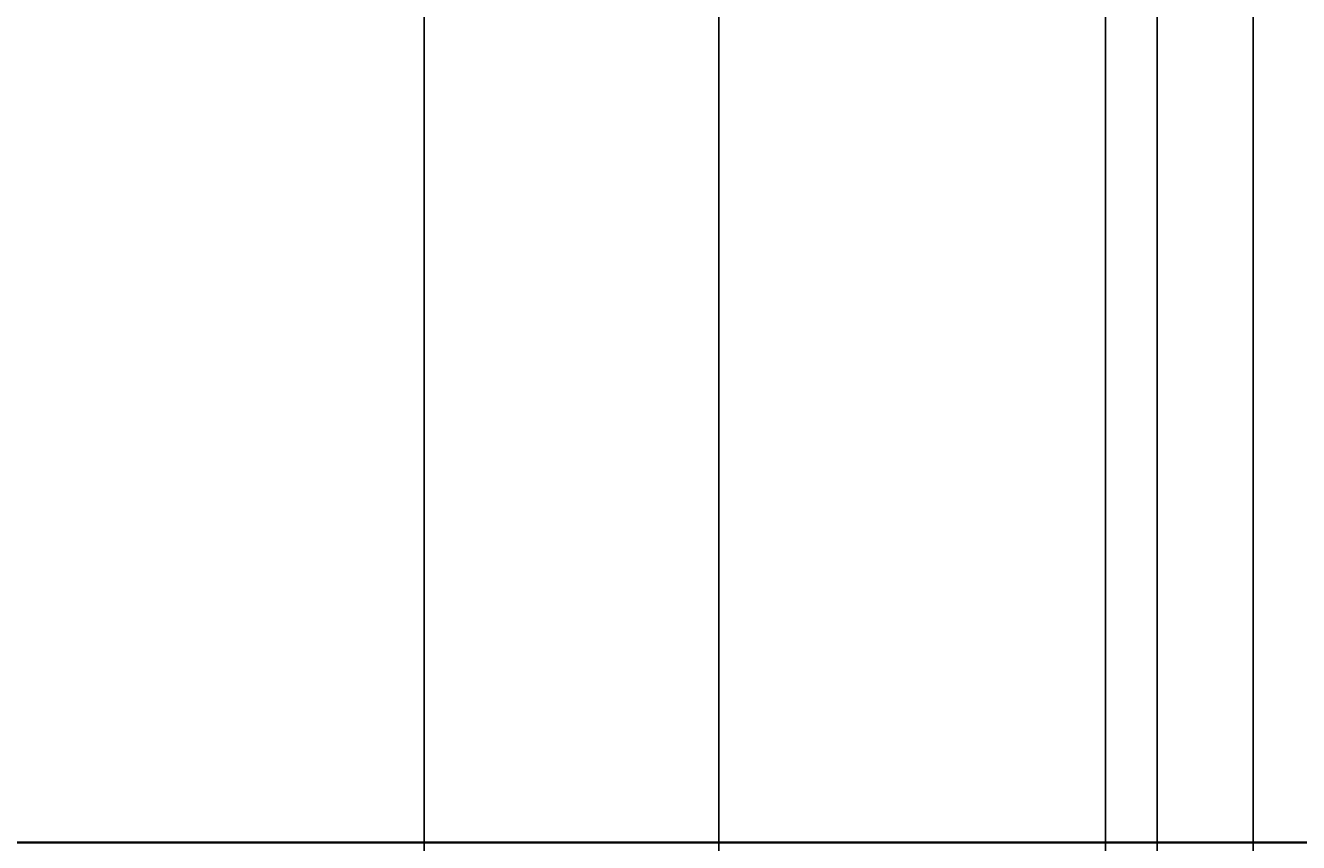
# Model space of a CAD drawing. Units: inches. Extents: x -6 to 289, y -8 to 323.
# Tile 96 of 107: x 222 to 248, y 259 to 276. Entities that reach past the tile are written whole.
import ezdxf

# ---------------------------------------------------------------- set-up
doc = ezdxf.new("R2010")
doc.units = ezdxf.units.IN
doc.header["$MEASUREMENT"] = 0
doc.layers.add('A-ANNO-DIMS', color=2, linetype='Continuous', lineweight=18)
doc.layers.add('A-ELEV', color=7, linetype='Continuous', lineweight=35)
doc.styles.get("Standard").update_dxf_attribs({"font": 'arial.ttf'})
doc.dimstyles.get("Standard").update_dxf_attribs({"dimtxt": 0.18, "dimasz": 0.18, "dimexe": 0.18, "dimexo": 0.0625, "dimgap": 0.09, "dimtad": 0, "dimtih": 1, "dimtoh": 1, "dimdec": 4, "dimzin": 0, "dimdsep": 46, "dimtxsty": 'Standard', "dimcen": 0.09, "dimadec": 0, "dimazin": 0, "dimtfac": 1, "dimtdec": 4, "dimtofl": 0, "dimtmove": 0, "dimatfit": 3, "dimfxl": 1, "dimtolj": 1, "dimtzin": 0, "dimarcsym": 0})

# ---------------------------------------------------------------- blocks, each defined once
blk = doc.blocks.new('*D13')
at = {"layer": 'A-ANNO-DIMS', "color": 0, "lineweight": -2, "transparency": 16777216}
for p, q in [((188.292, 226.951), (188.292, 322.969)), ((236.292, 226.951), (236.292, 322.969)), ((188.472, 322.789), (212.069, 322.789)), ((236.112, 322.789), (212.515, 322.789))]:
    blk.add_line(p, q, dxfattribs=at)
at = {"layer": 'A-ANNO-DIMS', "color": 0, "transparency": 16777216}
for points in [[(188.472, 322.819), (188.472, 322.759), (188.292, 322.789)], [(236.112, 322.819), (236.112, 322.759), (236.292, 322.789)]]:
    blk.add_solid(points, dxfattribs=at)
at = {"layer": 'Defpoints', "color": 0, "transparency": 16777216}
for p in [(236.292, 322.789), (188.292, 226.889), (236.292, 226.889)]:
    blk.add_point(p, dxfattribs=at)
at = {"layer": 'A-ANNO-DIMS', "color": 0, "transparency": 16777216, "insert": (212.292, 322.789), "char_height": 0.18, "attachment_point": 5}
blk.add_mtext('\\A1;48', dxfattribs=at)
blk = doc.blocks.new('*D14')
at = {"layer": 'A-ANNO-DIMS', "color": 0, "lineweight": -2, "transparency": 16777216}
for p, q in [((236.292, 226.951), (236.292, 322.969)), ((247.164, 162.411), (247.164, 322.969)), ((236.472, 322.789), (241.274, 322.789)), ((246.984, 322.789), (242.182, 322.789))]:
    blk.add_line(p, q, dxfattribs=at)
at = {"layer": 'A-ANNO-DIMS', "color": 0, "transparency": 16777216}
for points in [[(236.472, 322.819), (236.472, 322.759), (236.292, 322.789)], [(246.984, 322.819), (246.984, 322.759), (247.164, 322.789)]]:
    blk.add_solid(points, dxfattribs=at)
at = {"layer": 'Defpoints', "color": 0, "transparency": 16777216}
for p in [(247.164, 322.789), (236.292, 226.889), (247.164, 162.348)]:
    blk.add_point(p, dxfattribs=at)
at = {"layer": 'A-ANNO-DIMS', "color": 0, "transparency": 16777216, "insert": (241.728, 322.789), "char_height": 0.18, "attachment_point": 5}
blk.add_mtext('\\A1;10.872', dxfattribs=at)
blk = doc.blocks.new('*D15')
at = {"layer": 'A-ANNO-DIMS', "color": 0, "lineweight": -2, "transparency": 16777216}
for p, q in [((247.164, 162.411), (247.164, 322.969)), ((271.164, 7.351), (271.164, 322.969)), ((247.344, 322.789), (258.944, 322.789)), ((270.984, 322.789), (259.384, 322.789))]:
    blk.add_line(p, q, dxfattribs=at)
at = {"layer": 'A-ANNO-DIMS', "color": 0, "transparency": 16777216}
for points in [[(247.344, 322.819), (247.344, 322.759), (247.164, 322.789)], [(270.984, 322.819), (270.984, 322.759), (271.164, 322.789)]]:
    blk.add_solid(points, dxfattribs=at)
at = {"layer": 'Defpoints', "color": 0, "transparency": 16777216}
for p in [(271.164, 322.789), (247.164, 162.348), (271.164, 7.289)]:
    blk.add_point(p, dxfattribs=at)
at = {"layer": 'A-ANNO-DIMS', "color": 0, "transparency": 16777216, "insert": (259.164, 322.789), "char_height": 0.18, "attachment_point": 5}
blk.add_mtext('\\A1;24', dxfattribs=at)
blk = doc.blocks.new('*D27')
at = {"layer": 'A-ANNO-DIMS', "color": 0, "lineweight": -2, "transparency": 16777216}
for p, q in [((19.226, 307.289), (288.653, 307.289)), ((288.473, 307.109), (288.473, 277.471)), ((288.473, 247.469), (288.473, 277.107)), ((247.226, 247.289), (288.653, 247.289))]:
    blk.add_line(p, q, dxfattribs=at)
at = {"layer": 'A-ANNO-DIMS', "color": 0, "transparency": 16777216}
for points in [[(288.443, 307.109), (288.503, 307.109), (288.473, 307.289)], [(288.443, 247.469), (288.503, 247.469), (288.473, 247.289)]]:
    blk.add_solid(points, dxfattribs=at)
at = {"layer": 'Defpoints', "color": 0, "transparency": 16777216}
for p in [(19.164, 307.289), (288.473, 307.289), (247.164, 247.289)]:
    blk.add_point(p, dxfattribs=at)
at = {"layer": 'A-ANNO-DIMS', "color": 0, "transparency": 16777216, "insert": (288.473, 277.289), "char_height": 0.18, "attachment_point": 5}
blk.add_mtext('\\A1;60', dxfattribs=at)
blk = doc.blocks.new('*D80')
at = {"layer": 'A-ANNO-DIMS', "color": 0, "lineweight": -2, "transparency": 16777216}
for p, q in [((188.292, 116.842), (188.292, 322.969)), ((230.292, 116.842), (230.292, 322.969)), ((188.472, 322.789), (209.07, 322.789)), ((230.112, 322.789), (209.513, 322.789))]:
    blk.add_line(p, q, dxfattribs=at)
at = {"layer": 'A-ANNO-DIMS', "color": 0, "transparency": 16777216}
for points in [[(188.472, 322.819), (188.472, 322.759), (188.292, 322.789)], [(230.112, 322.819), (230.112, 322.759), (230.292, 322.789)]]:
    blk.add_solid(points, dxfattribs=at)
at = {"layer": 'Defpoints', "color": 0, "transparency": 16777216}
for p in [(230.292, 322.789), (188.292, 116.779), (230.292, 116.779)]:
    blk.add_point(p, dxfattribs=at)
at = {"layer": 'A-ANNO-DIMS', "color": 0, "transparency": 16777216, "insert": (209.292, 322.789), "char_height": 0.18, "attachment_point": 5}
blk.add_mtext('\\A1;42', dxfattribs=at)
blk = doc.blocks.new('*D81')
at = {"layer": 'A-ANNO-DIMS', "color": 0, "lineweight": -2, "transparency": 16777216}
for p, q in [((230.292, 68.842), (230.292, 322.969)), ((245.215, 66.286), (245.215, 322.969)), ((230.472, 322.789), (237.298, 322.789)), ((245.035, 322.789), (238.208, 322.789))]:
    blk.add_line(p, q, dxfattribs=at)
at = {"layer": 'A-ANNO-DIMS', "color": 0, "transparency": 16777216}
for points in [[(230.472, 322.819), (230.472, 322.759), (230.292, 322.789)], [(245.035, 322.819), (245.035, 322.759), (245.215, 322.789)]]:
    blk.add_solid(points, dxfattribs=at)
at = {"layer": 'Defpoints', "color": 0, "transparency": 16777216}
for p in [(245.215, 322.789), (230.292, 68.779), (245.215, 66.224)]:
    blk.add_point(p, dxfattribs=at)
at = {"layer": 'A-ANNO-DIMS', "color": 0, "transparency": 16777216, "insert": (237.753, 322.789), "char_height": 0.18, "attachment_point": 5}
blk.add_mtext('\\A1;14.923', dxfattribs=at)
blk = doc.blocks.new('*D82')
at = {"layer": 'A-ANNO-DIMS', "color": 0, "lineweight": -2, "transparency": 16777216}
for p, q in [((245.215, 66.286), (245.215, 322.969)), ((272.973, 66.286), (272.973, 322.969)), ((245.395, 322.789), (258.699, 322.789)), ((272.793, 322.789), (259.489, 322.789))]:
    blk.add_line(p, q, dxfattribs=at)
at = {"layer": 'A-ANNO-DIMS', "color": 0, "transparency": 16777216}
for points in [[(245.395, 322.819), (245.395, 322.759), (245.215, 322.789)], [(272.793, 322.819), (272.793, 322.759), (272.973, 322.789)]]:
    blk.add_solid(points, dxfattribs=at)
at = {"layer": 'Defpoints', "color": 0, "transparency": 16777216}
for p in [(272.973, 322.789), (245.215, 66.224), (272.973, 66.224)]:
    blk.add_point(p, dxfattribs=at)
at = {"layer": 'A-ANNO-DIMS', "color": 0, "transparency": 16777216, "insert": (259.094, 322.789), "char_height": 0.18, "attachment_point": 5}
blk.add_mtext('\\A1;27.76', dxfattribs=at)
blk = doc.blocks.new('*D98')
at = {"layer": 'A-ANNO-DIMS', "color": 0, "lineweight": -2, "transparency": 16777216}
for p, q in [((202.741, 159.411), (202.741, 322.969)), ((244.164, 159.411), (244.164, 322.969)), ((202.921, 322.789), (223.056, 322.789)), ((243.984, 322.789), (223.849, 322.789))]:
    blk.add_line(p, q, dxfattribs=at)
at = {"layer": 'A-ANNO-DIMS', "color": 0, "transparency": 16777216}
for points in [[(202.921, 322.819), (202.921, 322.759), (202.741, 322.789)], [(243.984, 322.819), (243.984, 322.759), (244.164, 322.789)]]:
    blk.add_solid(points, dxfattribs=at)
at = {"layer": 'Defpoints', "color": 0, "transparency": 16777216}
for p in [(244.164, 322.789), (202.741, 159.348), (244.164, 159.348)]:
    blk.add_point(p, dxfattribs=at)
at = {"layer": 'A-ANNO-DIMS', "color": 0, "transparency": 16777216, "insert": (223.452, 322.789), "char_height": 0.18, "attachment_point": 5}
blk.add_mtext('\\A1;41.42', dxfattribs=at)
blk = doc.blocks.new('*D99')
at = {"layer": 'A-ANNO-DIMS', "color": 0, "lineweight": -2, "transparency": 16777216}
for p, q in [((244.164, 159.411), (244.164, 322.969)), ((247.164, 162.411), (247.164, 322.969)), ((244.344, 322.789), (245.515, 322.789)), ((246.984, 322.789), (245.813, 322.789))]:
    blk.add_line(p, q, dxfattribs=at)
at = {"layer": 'A-ANNO-DIMS', "color": 0, "transparency": 16777216}
for points in [[(244.344, 322.819), (244.344, 322.759), (244.164, 322.789)], [(246.984, 322.819), (246.984, 322.759), (247.164, 322.789)]]:
    blk.add_solid(points, dxfattribs=at)
at = {"layer": 'Defpoints', "color": 0, "transparency": 16777216}
for p in [(247.164, 322.789), (247.164, 162.348), (244.164, 159.348)]:
    blk.add_point(p, dxfattribs=at)
at = {"layer": 'A-ANNO-DIMS', "color": 0, "transparency": 16777216, "insert": (245.664, 322.789), "char_height": 0.18, "attachment_point": 5}
blk.add_mtext('\\A1;3', dxfattribs=at)
blk = doc.blocks.new('*D100')
at = {"layer": 'A-ANNO-DIMS', "color": 0, "lineweight": -2, "transparency": 16777216}
for p, q in [((247.164, 162.411), (247.164, 322.969)), ((259.164, 139.351), (259.164, 322.969)), ((247.344, 322.789), (252.954, 322.789)), ((258.984, 322.789), (253.373, 322.789))]:
    blk.add_line(p, q, dxfattribs=at)
at = {"layer": 'A-ANNO-DIMS', "color": 0, "transparency": 16777216}
for points in [[(247.344, 322.819), (247.344, 322.759), (247.164, 322.789)], [(258.984, 322.819), (258.984, 322.759), (259.164, 322.789)]]:
    blk.add_solid(points, dxfattribs=at)
at = {"layer": 'Defpoints', "color": 0, "transparency": 16777216}
for p in [(259.164, 322.789), (247.164, 162.348), (259.164, 139.289)]:
    blk.add_point(p, dxfattribs=at)
at = {"layer": 'A-ANNO-DIMS', "color": 0, "transparency": 16777216, "insert": (253.164, 322.789), "char_height": 0.18, "attachment_point": 5}
blk.add_mtext('\\A1;12', dxfattribs=at)

msp = doc.modelspace()

# ---------------------------------------------------------------- linework, layer by layer
at = {"layer": 'A-ELEV'}
msp.add_line((115.1638, 259.2888), (271.1638, 259.2888), dxfattribs=at)

# ---------------------------------------------------------------- dimensions: what is measured, and where the dimension line sits
at = {"layer": 'A-ANNO-DIMS'}
for base, p1, p2, override, picture, middle in [((236.2918, 322.7888), (188.2918, 226.8887), (236.2918, 226.8887), {"dimdec": 0, "dimlfac": 1, "dimrnd": 0, "dimzin": 0, "dimdsep": 46, "dimlunit": 2}, '*D13', (212.2918, 322.7888)), ((230.2918, 322.7888), (188.2918, 116.7795), (230.2918, 116.7795), {"dimdec": 0, "dimlfac": 1, "dimrnd": 0, "dimzin": 0, "dimdsep": 46, "dimlunit": 2}, '*D80', (209.2918, 322.7888)), ((244.1638, 322.7888), (202.741, 159.3484), (244.1638, 159.3484), {"dimdec": 2, "dimlfac": 1, "dimrnd": 0, "dimzin": 0, "dimdsep": 46, "dimlunit": 2}, '*D98', (223.4524, 322.7888)), ((245.2146, 322.7888), (230.2918, 68.7795), (245.2146, 66.2238), {"dimdec": 3, "dimlfac": 1, "dimrnd": 0, "dimzin": 0, "dimdsep": 46, "dimlunit": 2}, '*D81', (237.7532, 322.7888)), ((247.1638, 322.7888), (236.2918, 226.8887), (247.1638, 162.3484), {"dimdec": 3, "dimlfac": 1, "dimrnd": 0, "dimzin": 0, "dimdsep": 46, "dimlunit": 2}, '*D14', (241.7278, 322.7888)), ((247.1638, 322.7888), (244.1638, 159.3484), (247.1638, 162.3484), {"dimdec": 0, "dimlfac": 1, "dimrnd": 0, "dimzin": 0, "dimdsep": 46, "dimlunit": 2}, '*D99', (245.6638, 322.7888)), ((272.9733, 322.7888), (245.2146, 66.2238), (272.9733, 66.2238), {"dimdec": 2, "dimlfac": 1, "dimrnd": 0, "dimzin": 0, "dimdsep": 46, "dimlunit": 2}, '*D82', (259.0939, 322.7888)), ((271.1638, 322.7888), (247.1638, 162.3484), (271.1638, 7.2888), {"dimdec": 0, "dimlfac": 1, "dimrnd": 0, "dimzin": 0, "dimdsep": 46, "dimlunit": 2}, '*D15', (259.1638, 322.7888)), ((259.1638, 322.7888), (247.1638, 162.3484), (259.1638, 139.2888), {"dimdec": 0, "dimlfac": 1, "dimrnd": 0, "dimzin": 0, "dimdsep": 46, "dimlunit": 2}, '*D100', (253.1638, 322.7888))]:
    dim = msp.add_linear_dim(base=base, p1=p1, p2=p2, dimstyle='Standard', override=override, dxfattribs=at)
    dim.commit()
    dim.dimension.update_dxf_attribs({"geometry": picture, "text_midpoint": middle})
dim = msp.add_linear_dim(base=(288.4733, 307.2888), p1=(247.1638, 247.2888), p2=(19.1638, 307.2888), angle=90, dimstyle='Standard', override={"dimdec": 0, "dimlfac": 1, "dimrnd": 0, "dimzin": 0, "dimdsep": 46, "dimlunit": 2}, dxfattribs=at)
dim.commit()
dim.dimension.update_dxf_attribs({"geometry": '*D27', "text_midpoint": (288.4733, 277.2888)})

doc.saveas('drawing.dxf')
